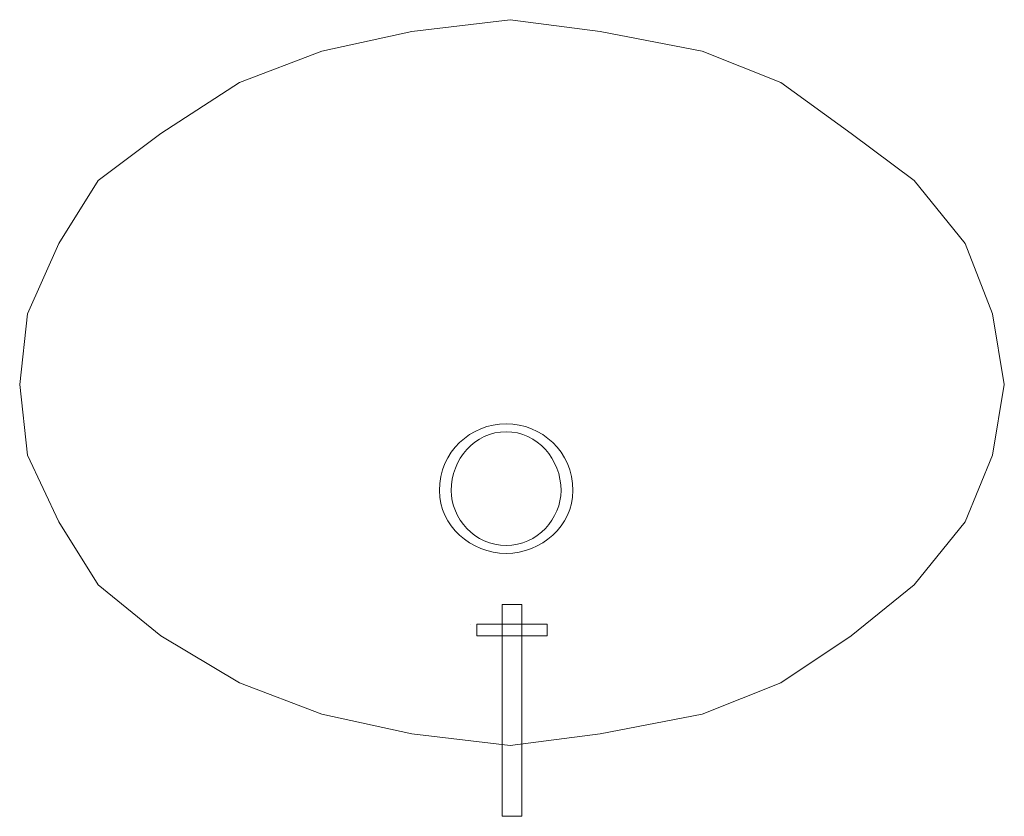
# Model space of a CAD drawing. Units: inches. Extents: x 79 to 8696167, y -3690578 to 147.
# Tile 9 of 10: x 3223832 to 3224047, y -28222 to -28048. Entities that reach past the tile are written whole.
import ezdxf

# ---------------------------------------------------------------- set-up
doc = ezdxf.new("R2010")
doc.units = ezdxf.units.IN
doc.header["$MEASUREMENT"] = 0
doc.layers.get('0').update_dxf_attribs({"color": 253})
doc.layers.add('PLUMBING FIXTURES', color=9, linetype='Continuous', lineweight=18)

# ---------------------------------------------------------------- blocks, each defined once
blk = doc.blocks.new('WASH')
for p, q in [((268674.713, -2306.293), (268675.07, -2306.293)), ((268674.249, -2306.864), (268674.249, -2306.65)), ((268675.535, -2306.864), (268675.535, -2306.65)), ((268674.713, -2310.15), (268675.07, -2310.15))]:
    blk.add_line(p, q)
for points in [[(268665.927, -2302.293), (268666.07, -2301.007), (268666.642, -2299.722), (268667.356, -2298.579), (268668.499, -2297.722), (268669.927, -2296.793), (268671.427, -2296.222), (268673.07, -2295.864), (268674.856, -2295.65), (268676.499, -2295.864), (268678.356, -2296.222), (268679.785, -2296.793), (268681.07, -2297.722), (268682.213, -2298.579), (268683.142, -2299.722), (268683.642, -2301.007), (268683.856, -2302.293), (268683.642, -2303.579), (268683.142, -2304.793), (268682.213, -2305.936), (268681.07, -2306.864), (268679.785, -2307.722), (268678.356, -2308.293), (268676.499, -2308.65), (268674.856, -2308.864), (268673.07, -2308.65), (268671.427, -2308.293), (268669.927, -2307.722), (268668.499, -2306.864), (268667.356, -2305.936), (268666.642, -2304.793), (268666.07, -2303.579)], [(268674.856, -2306.293), (268674.856, -2306.293)], [(268674.142, -2306.65), (268674.142, -2306.65)], [(268675.427, -2306.65), (268675.427, -2306.65)]]:
    blk.add_lwpolyline(points, close=True)
for points in [[(268674.713, -2310.15), (268674.713, -2306.293), (268674.713, -2306.293)], [(268675.07, -2310.15), (268675.07, -2306.293), (268675.07, -2306.293)], [(268674.249, -2306.65), (268675.535, -2306.65), (268675.535, -2306.65)], [(268674.249, -2306.864), (268675.535, -2306.864), (268675.535, -2306.864)]]:
    blk.add_lwpolyline(points)
for points in [[(268673.57, -2304.222), (268673.57, -2304.864), (268674.142, -2305.364), (268674.785, -2305.364), (268674.785, -2305.364), (268675.427, -2305.364), (268675.999, -2304.864), (268675.999, -2304.222), (268675.999, -2304.222), (268675.999, -2303.507), (268675.427, -2303.007), (268674.785, -2303.007), (268674.785, -2303.007), (268674.142, -2303.007), (268673.57, -2303.507), (268673.57, -2304.222)], [(268673.785, -2304.222), (268673.785, -2304.722), (268674.213, -2305.222), (268674.785, -2305.222), (268674.785, -2305.222), (268675.356, -2305.222), (268675.785, -2304.722), (268675.785, -2304.222), (268675.785, -2304.222), (268675.785, -2303.65), (268675.356, -2303.15), (268674.785, -2303.15), (268674.785, -2303.15), (268674.213, -2303.15), (268673.785, -2303.65), (268673.785, -2304.222)]]:
    blk.add_open_spline(points, degree=3, knots=[0, 0, 0, 0, 0.0625, 0.0625, 0.0625, 0.062501, 0.125, 0.125, 0.125, 0.125001, 0.1875, 0.1875, 0.1875, 0.187501, 1, 1, 1, 1])

msp = doc.modelspace()

# ---------------------------------------------------------------- block references
at = {"layer": 'PLUMBING FIXTURES', "xscale": 12, "yscale": 12, "zscale": 12}
msp.add_blockref('WASH', (-159.348, -499.792), dxfattribs=at)

doc.saveas('drawing.dxf')
